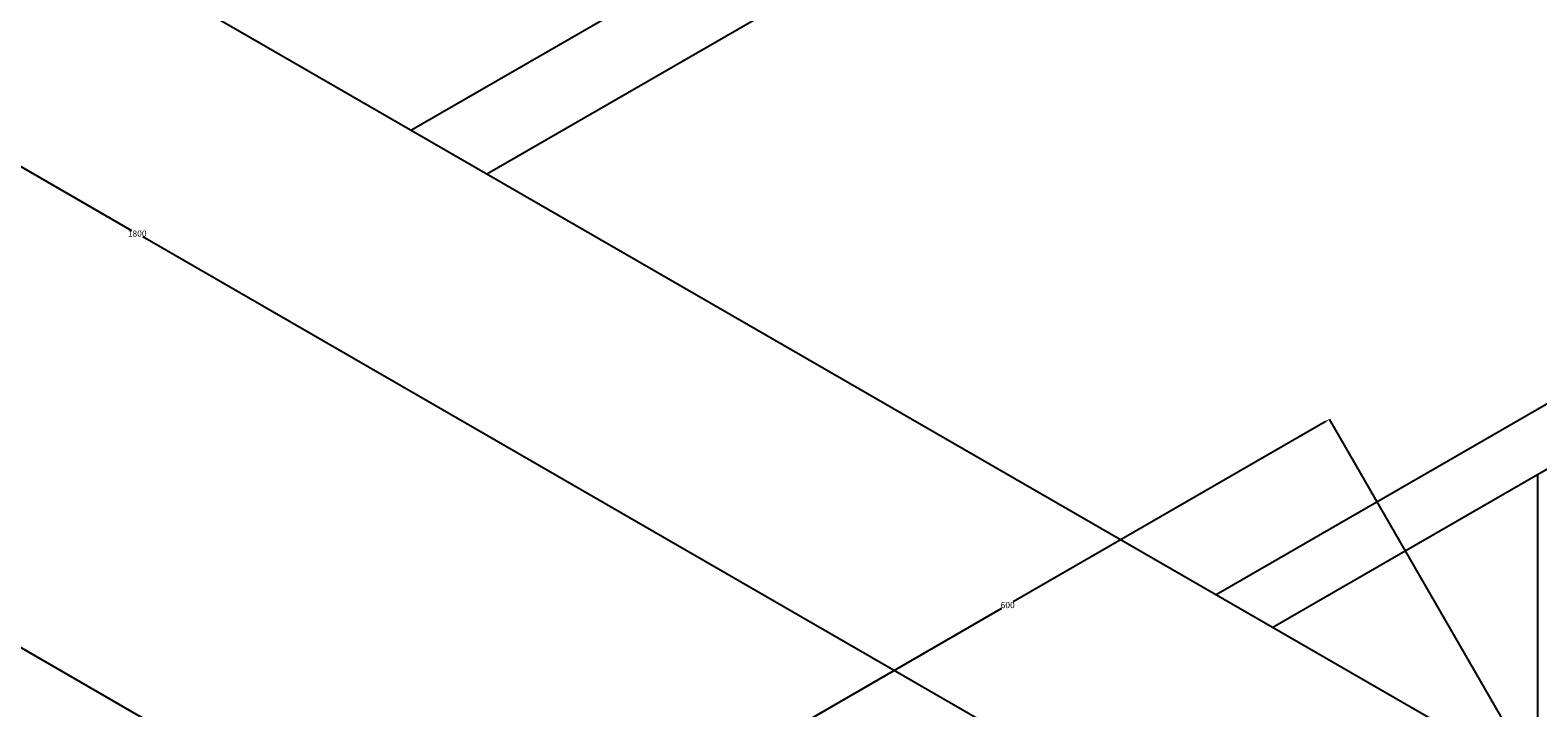
# Model space of a CAD drawing. Units: metres. Extents: x -2391 to 4922, y -635 to 4845.
# Tile 18 of 37: x -1186 to 31, y 2464 to 3011. Entities that reach past the tile are written whole.
import ezdxf

# ---------------------------------------------------------------- set-up
doc = ezdxf.new("R2010")
doc.units = ezdxf.units.M
doc.header["$MEASUREMENT"] = 0
doc.layers.add('A-ANNO-DIMS', color=2, linetype='Continuous', lineweight=18)
doc.layers.add('A-FLOR-FIXT', color=3, linetype='Continuous', lineweight=25)
doc.styles.get("Standard").update_dxf_attribs({"font": 'arial.ttf'})
doc.dimstyles.get("Standard").update_dxf_attribs({"dimtxt": 5, "dimasz": 4, "dimexe": 0.18, "dimexo": 0.0625, "dimgap": 0.09, "dimtad": 0, "dimtih": 1, "dimtoh": 1, "dimdec": 0, "dimzin": 0, "dimdsep": 46, "dimtxsty": 'Standard', "dimcen": 0.09, "dimadec": 0, "dimazin": 0, "dimtfac": 1, "dimtdec": 0, "dimtofl": 0, "dimtmove": 0, "dimatfit": 3, "dimfxl": 1, "dimtolj": 1, "dimtzin": 0, "dimarcsym": 0})

# ---------------------------------------------------------------- blocks, each defined once
blk = doc.blocks.new('*D8')
at = {"layer": 'A-ANNO-DIMS', "color": 0, "lineweight": -2, "transparency": 16777216}
for p, q in [((-2047.3, 3005.2), (-2047.3, -631.4)), ((4577.8, 2350.2), (4577.8, -631.4)), ((-2043.3, -631.2), (1257.6, -631.2)), ((4573.8, -631.2), (1272.8, -631.2))]:
    blk.add_line(p, q, dxfattribs=at)
at = {"layer": 'A-ANNO-DIMS', "color": 0, "transparency": 16777216}
for points in [[(-2043.3, -630.6), (-2043.3, -631.9), (-2047.3, -631.2)], [(4573.8, -630.6), (4573.8, -631.9), (4577.8, -631.2)]]:
    blk.add_solid(points, dxfattribs=at)
at = {"layer": 'Defpoints', "color": 0, "transparency": 16777216}
for p in [(-2047.3, 3005.3), (4577.8, 2350.3), (4577.8, -631.2)]:
    blk.add_point(p, dxfattribs=at)
at = {"layer": 'A-ANNO-DIMS', "color": 0, "transparency": 16777216, "insert": (1265.2, -631.2), "char_height": 5, "attachment_point": 5}
blk.add_mtext('\\A1;6625', dxfattribs=at)
blk = doc.blocks.new('*D9')
at = {"layer": 'A-ANNO-DIMS', "color": 0, "lineweight": -2, "transparency": 16777216}
for p, q in [((-2047.3, 3005.3), (-2047.3, 4842)), ((-2043.3, 4841.8), (-755.9, 4841.8)), ((546.7, 4841.8), (-740.7, 4841.8)), ((550.7, 4505.3), (550.7, 4842))]:
    blk.add_line(p, q, dxfattribs=at)
at = {"layer": 'A-ANNO-DIMS', "color": 0, "transparency": 16777216}
for points in [[(-2043.3, 4842.4), (-2043.3, 4841.1), (-2047.3, 4841.8)], [(546.7, 4842.4), (546.7, 4841.1), (550.7, 4841.8)]]:
    blk.add_solid(points, dxfattribs=at)
at = {"layer": 'Defpoints', "color": 0, "transparency": 16777216}
for p in [(550.7, 4841.8), (550.7, 4505.3), (-2047.3, 3005.3)]:
    blk.add_point(p, dxfattribs=at)
at = {"layer": 'A-ANNO-DIMS', "color": 0, "transparency": 16777216, "insert": (-748.3, 4841.8), "char_height": 5, "attachment_point": 5}
blk.add_mtext('\\A1;2598', dxfattribs=at)
blk = doc.blocks.new('*D10')
at = {"layer": 'A-ANNO-DIMS', "color": 0, "lineweight": -2, "transparency": 16777216}
for p, q in [((550.7, 4505.3), (-2384, 4505.3)), ((-2383.8, 4501.3), (-2383.8, 2107.9)), ((-2383.8, -290.7), (-2383.8, 2102.6)), ((-488.6, -294.7), (-2384, -294.7))]:
    blk.add_line(p, q, dxfattribs=at)
at = {"layer": 'A-ANNO-DIMS', "color": 0, "transparency": 16777216}
for points in [[(-2384.5, 4501.3), (-2383.2, 4501.3), (-2383.8, 4505.3)], [(-2384.5, -290.7), (-2383.2, -290.7), (-2383.8, -294.7)]]:
    blk.add_solid(points, dxfattribs=at)
at = {"layer": 'Defpoints', "color": 0, "transparency": 16777216}
for p in [(-2383.8, 4505.3), (550.7, 4505.3), (-488.5, -294.7)]:
    blk.add_point(p, dxfattribs=at)
at = {"layer": 'A-ANNO-DIMS', "color": 0, "transparency": 16777216, "insert": (-2383.8, 2105.3), "char_height": 5, "attachment_point": 5}
blk.add_mtext('\\A1;4800', dxfattribs=at)
blk = doc.blocks.new('*D41')
at = {"layer": 'A-ANNO-DIMS', "color": 0, "lineweight": -2, "transparency": 16777216}
for p, q in [((-2047.3, 3005.3), (-1879, 3296.8)), ((-1875.6, 3294.7), (-1104.2, 2849.3)), ((-323.7, 2398.7), (-1095.1, 2844.1)), ((-488.5, 2105.3), (-320.1, 2396.8))]:
    blk.add_line(p, q, dxfattribs=at)
at = {"layer": 'A-ANNO-DIMS', "color": 0, "transparency": 16777216}
for points in [[(-1875.3, 3295.3), (-1876, 3294.1), (-1879.1, 3296.7)], [(-323.4, 2399.3), (-324, 2398.1), (-320.2, 2396.7)]]:
    blk.add_solid(points, dxfattribs=at)
at = {"layer": 'Defpoints', "color": 0, "transparency": 16777216}
for p in [(-2047.3, 3005.3), (-320.2, 2396.7), (-488.5, 2105.3)]:
    blk.add_point(p, dxfattribs=at)
at = {"layer": 'A-ANNO-DIMS', "color": 0, "transparency": 16777216, "insert": (-1099.7, 2846.7), "char_height": 5, "attachment_point": 5}
blk.add_mtext('\\A1;1800', dxfattribs=at)
blk = doc.blocks.new('*D42')
at = {"layer": 'A-ANNO-DIMS', "color": 0, "lineweight": -2, "transparency": 16777216}
for p, q in [((-140.6, 2694.7), (-392.4, 2549.3)), ((31.1, 2405.3), (-137.2, 2696.8)), ((-653.3, 2398.7), (-401.5, 2544.1)), ((-488.5, 2105.3), (-656.8, 2396.8))]:
    blk.add_line(p, q, dxfattribs=at)
at = {"layer": 'A-ANNO-DIMS', "color": 0, "transparency": 16777216}
for points in [[(-140.9, 2695.3), (-140.3, 2694.1), (-137.1, 2696.7)], [(-653.6, 2399.3), (-652.9, 2398.1), (-656.7, 2396.7)]]:
    blk.add_solid(points, dxfattribs=at)
at = {"layer": 'Defpoints', "color": 0, "transparency": 16777216}
for p in [(-137.1, 2696.7), (31.1, 2405.3), (-488.5, 2105.3)]:
    blk.add_point(p, dxfattribs=at)
at = {"layer": 'A-ANNO-DIMS', "color": 0, "transparency": 16777216, "insert": (-396.9, 2546.7), "char_height": 5, "attachment_point": 5}
blk.add_mtext('\\A1;600', dxfattribs=at)

msp = doc.modelspace()

# ---------------------------------------------------------------- linework, layer by layer
at = {"layer": 'A-FLOR-FIXT'}
for p, q in [((612.0233, 3790.6571), (-878.2, 2930.2763)), ((612.0233, 3719.8954), (-816.9186, 2894.8954)), ((-1527.7191, 3305.2763), (31.1266, 2405.2763)), ((-2047.3343, 3005.2763), (-488.4886, 2105.2763)), ((-228.681, 2555.2763), (550.7419, 3005.2763)), ((-182.857, 2528.8198), (546.8938, 2950.1416)), ((31.1266, 1825.2763), (31.1266, 2652.3633))]:
    msp.add_line(p, q, dxfattribs=at)

# ---------------------------------------------------------------- dimensions: what is measured, and where the dimension line sits
at = {"layer": 'A-ANNO-DIMS'}
for base, p2, picture, middle in [((550.7419, 4841.7763), (550.7419, 4505.2763), '*D9', (-748.2962, 4841.7763)), ((4577.76, -631.2237), (4577.76, 2350.2763), '*D8', (1265.2128, -631.2237))]:
    dim = msp.add_linear_dim(base=base, p1=(-2047.3343, 3005.2763), p2=p2, dimstyle='Standard', override={"dimdec": 0, "dimlfac": 1, "dimrnd": 0, "dimzin": 0, "dimdsep": 46, "dimlunit": 2}, dxfattribs=at)
    dim.commit()
    dim.dimension.update_dxf_attribs({"geometry": picture, "text_midpoint": middle})
for base, p1, p2, angle, picture, middle in [((-2383.8343, 4505.2763), (-488.4886, -294.7237), (550.7419, 4505.2763), 90, '*D10', (-2383.8343, 2105.2763)), ((-320.2386, 2396.6938), (-2047.3343, 3005.2763), (-488.4886, 2105.2763), 330, '*D41', (-1099.6615, 2846.6938)), ((-137.1234, 2696.6938), (-488.4886, 2105.2763), (31.1266, 2405.2763), 30, '*D42', (-396.931, 2546.6938))]:
    dim = msp.add_linear_dim(base=base, p1=p1, p2=p2, angle=angle, dimstyle='Standard', override={"dimdec": 0, "dimlfac": 1, "dimrnd": 0, "dimzin": 0, "dimdsep": 46, "dimlunit": 2}, dxfattribs=at)
    dim.commit()
    dim.dimension.update_dxf_attribs({"geometry": picture, "text_midpoint": middle})

doc.saveas('drawing.dxf')
